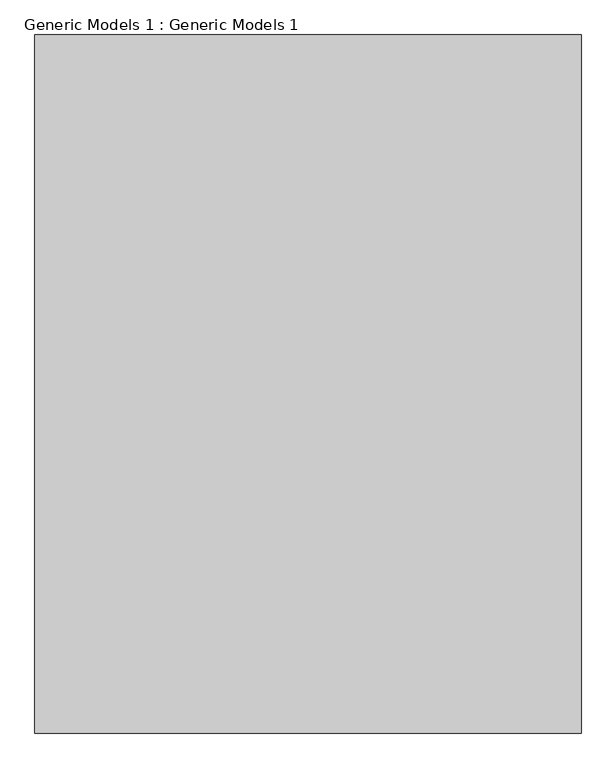
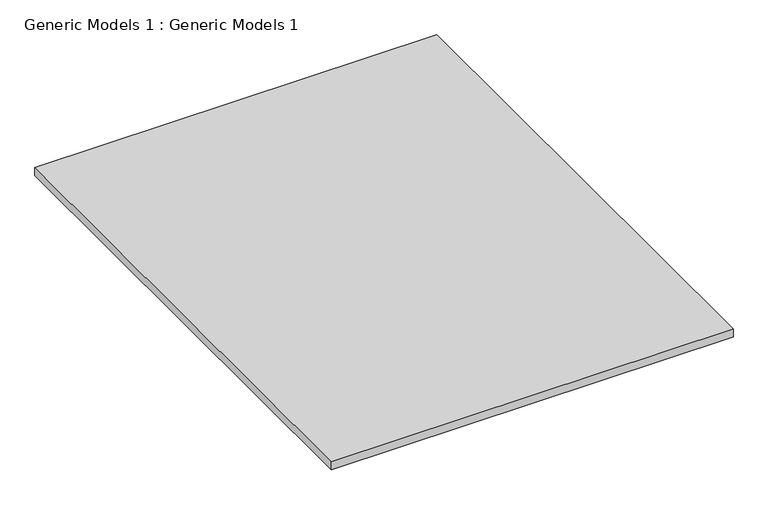
"""IFC4 building model written with IfcOpenShell, lengths in millimetres: proxy geometry, Generic Models 1 : Generic Models 1."""

from ifc_helpers import new_model, si_unit, frame, origin, place, context, project, spatial, polyline, outline, extrude, source, transform, mapped, element, save


def generic_models_1_generic_models_1_2a073142(model_context):
    return source(origin(), model_context, "Body", "SweptSolid", [
        extrude(outline(polyline([(-3888.4267684, 1817.9931613), (-3888.4267684, -17207.0242702), (-18783.334105, -17207.0242702), (-18783.334105, 1817.9931613), (-3888.4267684, 1817.9931613)])), frame((0.0, 0.0, -304.8), z_axis=(0.0, 0.0, 1.0), x_axis=(1.0, 0.0, 0.0)), (0.0, 0.0, 1.0), 304.8),
    ])


if __name__ == "__main__":
    model = new_model("IFC4")
    model_context = context("Model", 3, world=origin())
    ifc_project = project(units=[si_unit("LENGTHUNIT", "METRE", prefix="MILLI")], contexts=[model_context])
    site = spatial("IfcSite", under=ifc_project)
    building = spatial("IfcBuilding", under=site)
    placement = place(None, origin())
    generic_models_1_generic_models_1_shape = generic_models_1_generic_models_1_2a073142(model_context)
    element("IfcBuildingElementProxy", 1, Name="Generic Models 1 : Generic Models 1", ObjectType="Generic Models 1 : Generic Models 1", at=placement, inside=building, context=model_context, shape_type="MappedRepresentation", body=[
        mapped(generic_models_1_generic_models_1_shape, transform((0.0, 0.0, 0.0), x_axis=(1.0, 0.0, 0.0), y_axis=(0.0, 1.0, 0.0), z_axis=(0.0, 0.0, 1.0))),
    ])
    save(model, "model.ifc")
